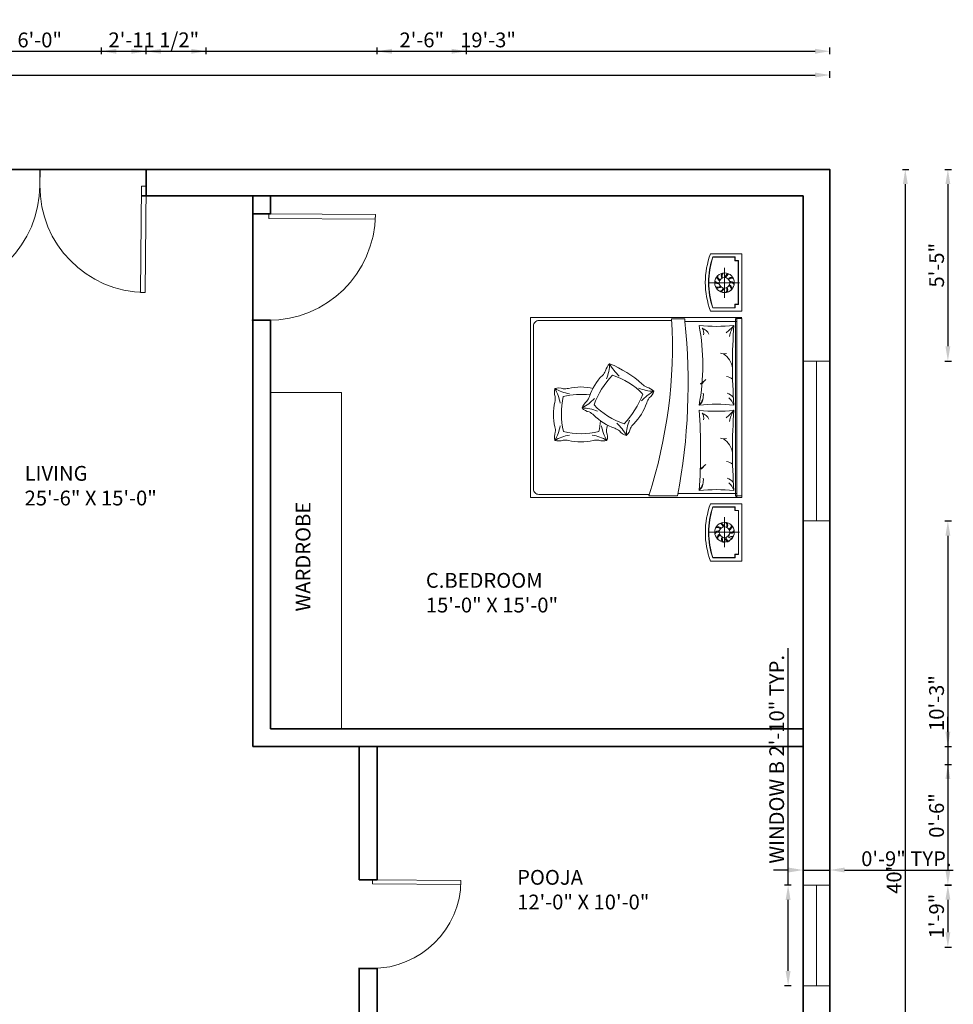
# Model space of a CAD drawing. Units: inches. Extents: x -100 to 766, y -562 to 63.
# Tile 11 of 11: x 448 to 763, y -269 to 63. Entities that reach past the tile are written whole.
import ezdxf

# ---------------------------------------------------------------- set-up
doc = ezdxf.new("R2010")
doc.units = ezdxf.units.IN
for name, color, linetype, lineweight in [('A-ANNO-DIMS', 2, 'Continuous', 18), ('A-ANNO-TEXT', 7, 'Continuous', 18), ('A-AREA-IDEN', 7, 'Continuous', 18), ('A-DOOR', 3, 'Continuous', 18), ('A-FLOR-CASE', 32, 'Continuous', 18), ('A-GLAZ', 4, 'Continuous', 18), ('A-WALL', 7, 'Continuous', 35), ('furn', 8, 'Continuous', 13)]:
    doc.layers.add(name, color=color, linetype=linetype, lineweight=lineweight)
doc.styles.get("Standard").update_dxf_attribs({"font": 'arial.ttf'})
doc.dimstyles.new('ISO-25', dxfattribs={"dimtxt": 5, "dimasz": 5, "dimexe": 1.25, "dimexo": 0.625, "dimtad": 1, "dimlunit": 3, "dimtxsty": 'Standard', "dimcen": 2.5, "dimadec": 0, "dimazin": 0, "dimtfac": 1, "dimtmove": 0, "dimatfit": 3, "dimfxl": 1, "dimfxlon": 1, "dimarcsym": 0})

# ---------------------------------------------------------------- blocks, each defined once
blk = doc.blocks.new('*U2')
for p, q in [((0, 0), (0, -6)), ((40, 0), (40, -6))]:
    blk.add_line(p, q)
blk.add_lwpolyline([(0, 0), (0, 40), (1.75, 40), (1.75, 0)], close=True)
blk.add_arc((0, 0), 40, 0, 90)
blk = doc.blocks.new('*D9')
at = {"layer": 'A-ANNO-DIMS', "color": 0, "lineweight": -2, "transparency": 16777216}
for p, q in [((1.39, 43.65), (1.39, 45.9)), ((6.39, 44.65), (716.39, 44.65)), ((721.39, 43.65), (721.39, 45.9))]:
    blk.add_line(p, q, dxfattribs=at)
at = {"layer": 'A-ANNO-DIMS', "color": 0, "transparency": 16777216}
for points in [[(6.39, 45.48), (6.39, 43.82), (1.39, 44.65)], [(716.39, 45.48), (716.39, 43.82), (721.39, 44.65)]]:
    blk.add_solid(points, dxfattribs=at)
at = {"layer": 'Defpoints', "color": 0, "transparency": 16777216}
for p in [(721.39, 44.65), (1.39, 12.79), (721.39, 12.79)]:
    blk.add_point(p, dxfattribs=at)
at = {"layer": 'A-ANNO-DIMS', "color": 0, "transparency": 16777216, "insert": (361.39, 47.83), "char_height": 5, "attachment_point": 5}
blk.add_mtext("60'", dxfattribs=at)
blk = doc.blocks.new('*D10')
at = {"layer": 'A-ANNO-DIMS', "color": 0, "lineweight": -2, "transparency": 16777216}
for p, q in [((745.89, 12.79), (748.14, 12.79)), ((746.89, 7.79), (746.89, -462.21)), ((745.89, -467.21), (748.14, -467.21))]:
    blk.add_line(p, q, dxfattribs=at)
at = {"layer": 'A-ANNO-DIMS', "color": 0, "transparency": 16777216}
for points in [[(746.06, 7.79), (747.73, 7.79), (746.89, 12.79)], [(746.06, -462.21), (747.73, -462.21), (746.89, -467.21)]]:
    blk.add_solid(points, dxfattribs=at)
at = {"layer": 'Defpoints', "color": 0, "transparency": 16777216}
for p in [(721.39, 12.79), (721.39, -467.21), (746.89, -467.21)]:
    blk.add_point(p, dxfattribs=at)
at = {"layer": 'A-ANNO-DIMS', "color": 0, "transparency": 16777216, "insert": (743.72, -227.21), "char_height": 5, "attachment_point": 5, "rotation": 90}
blk.add_mtext("40'", dxfattribs=at)
blk = doc.blocks.new('WIN-54IN')
blk.add_line((4.5, 54), (4.5, 0))
blk.add_lwpolyline([(0, 54), (9, 54), (9, 0), (0, 0)], close=True)
blk = doc.blocks.new('WIN-34IN')
blk.add_line((4.5, 34), (4.5, 0))
blk.add_lwpolyline([(0, 34), (9, 34), (9, 0), (0, 0)], close=True)
blk = doc.blocks.new('*D20')
at = {"layer": 'A-ANNO-DIMS', "color": 0, "lineweight": -2, "transparency": 16777216}
for p, q in [((707.29, -229.01), (707.29, -149.01)), ((708.29, -229.01), (706.04, -229.01)), ((707.29, -258.01), (707.29, -234.01)), ((708.29, -263.01), (706.04, -263.01))]:
    blk.add_line(p, q, dxfattribs=at)
at = {"layer": 'A-ANNO-DIMS', "color": 0, "transparency": 16777216}
for points in [[(706.45, -234.01), (708.12, -234.01), (707.29, -229.01)], [(706.45, -258.01), (708.12, -258.01), (707.29, -263.01)]]:
    blk.add_solid(points, dxfattribs=at)
at = {"layer": 'Defpoints', "color": 0, "transparency": 16777216}
for p in [(707.29, -229.01), (712.39, -229.01), (712.39, -263.01)]:
    blk.add_point(p, dxfattribs=at)
at = {"layer": 'A-ANNO-DIMS', "color": 0, "transparency": 16777216, "insert": (704.08, -186.51), "char_height": 5, "attachment_point": 5, "rotation": 90}
blk.add_mtext('WINDOW B 2\'-10" TYP.', dxfattribs=at)
blk = doc.blocks.new('*D21')
at = {"layer": 'A-ANNO-DIMS', "color": 0, "lineweight": -2, "transparency": 16777216}
for p, q in [((712.39, -224.91), (712.39, -222.66)), ((721.39, -224.91), (721.39, -222.66)), ((707.39, -223.91), (702.39, -223.91)), ((712.39, -223.91), (721.39, -223.91)), ((726.39, -223.91), (763.12, -223.91))]:
    blk.add_line(p, q, dxfattribs=at)
at = {"layer": 'A-ANNO-DIMS', "color": 0, "transparency": 16777216}
for points in [[(707.39, -223.08), (707.39, -224.75), (712.39, -223.91)], [(726.39, -223.08), (726.39, -224.75), (721.39, -223.91)]]:
    blk.add_solid(points, dxfattribs=at)
at = {"layer": 'Defpoints', "color": 0, "transparency": 16777216}
for p in [(721.39, -223.91), (712.39, -229.01), (721.39, -229.01)]:
    blk.add_point(p, dxfattribs=at)
at = {"layer": 'A-ANNO-DIMS', "color": 0, "transparency": 16777216, "insert": (747.25, -220.74), "char_height": 5, "attachment_point": 5}
blk.add_mtext('0\'-9" TYP.', dxfattribs=at)
blk = doc.blocks.new('*D44')
at = {"layer": 'A-ANNO-DIMS', "color": 0, "lineweight": -2, "transparency": 16777216}
for p, q in [((418.39, 51.68), (418.39, 53.93)), ((490.39, 51.68), (490.39, 53.93)), ((423.39, 52.68), (485.39, 52.68))]:
    blk.add_line(p, q, dxfattribs=at)
at = {"layer": 'A-ANNO-DIMS', "color": 0, "transparency": 16777216}
for points in [[(423.39, 53.51), (423.39, 51.84), (418.39, 52.68)], [(485.39, 53.51), (485.39, 51.84), (490.39, 52.68)]]:
    blk.add_solid(points, dxfattribs=at)
at = {"layer": 'Defpoints', "color": 0, "transparency": 16777216}
for p in [(490.39, 52.68), (418.39, 12.79), (490.39, 12.79)]:
    blk.add_point(p, dxfattribs=at)
at = {"layer": 'A-ANNO-DIMS', "color": 0, "transparency": 16777216, "insert": (454.39, 55.86), "char_height": 5, "attachment_point": 5}
blk.add_mtext('6\'-0"', dxfattribs=at)
blk = doc.blocks.new('*D45')
at = {"layer": 'A-ANNO-DIMS', "color": 0, "lineweight": -2, "transparency": 16777216}
for p, q in [((490.39, 51.68), (490.39, 53.93)), ((721.39, 51.68), (721.39, 53.93)), ((495.39, 52.68), (716.39, 52.68))]:
    blk.add_line(p, q, dxfattribs=at)
at = {"layer": 'A-ANNO-DIMS', "color": 0, "transparency": 16777216}
for points in [[(495.39, 53.51), (495.39, 51.84), (490.39, 52.68)], [(716.39, 53.51), (716.39, 51.84), (721.39, 52.68)]]:
    blk.add_solid(points, dxfattribs=at)
at = {"layer": 'Defpoints', "color": 0, "transparency": 16777216}
for p in [(721.39, 52.68), (490.39, 12.79), (721.39, 12.79)]:
    blk.add_point(p, dxfattribs=at)
at = {"layer": 'A-ANNO-DIMS', "color": 0, "transparency": 16777216, "insert": (605.89, 55.86), "char_height": 5, "attachment_point": 5}
blk.add_mtext('19\'-3"', dxfattribs=at)
blk = doc.blocks.new('*D48')
at = {"layer": 'A-ANNO-DIMS', "color": 0, "lineweight": -2, "transparency": 16777216}
for p, q in [((-88.51, -227.21), (-90.76, -227.21)), ((-89.51, -232.21), (-89.51, -252.21)), ((-88.51, -257.21), (-90.76, -257.21))]:
    blk.add_line(p, q, dxfattribs=at)
at = {"layer": 'A-ANNO-DIMS', "color": 0, "transparency": 16777216}
for points in [[(-90.35, -232.21), (-88.68, -232.21), (-89.51, -227.21)], [(-90.35, -252.21), (-88.68, -252.21), (-89.51, -257.21)]]:
    blk.add_solid(points, dxfattribs=at)
at = {"layer": 'Defpoints', "color": 0, "transparency": 16777216}
for p in [(562.39, -227.21), (-89.51, -257.21), (562.39, -257.21)]:
    blk.add_point(p, dxfattribs=at)
at = {"layer": 'A-ANNO-DIMS', "color": 0, "transparency": 16777216, "insert": (-92.69, -242.21), "char_height": 5, "attachment_point": 5, "rotation": 90}
blk.add_mtext('2\'-6"', dxfattribs=at)
blk = doc.blocks.new('*D52')
at = {"layer": 'A-ANNO-DIMS', "color": 0, "lineweight": -2, "transparency": 16777216}
for p, q in [((568.39, 51.68), (568.39, 53.93)), ((598.6, 51.68), (598.6, 53.93)), ((573.39, 52.68), (593.6, 52.68))]:
    blk.add_line(p, q, dxfattribs=at)
at = {"layer": 'A-ANNO-DIMS', "color": 0, "transparency": 16777216}
for points in [[(573.39, 53.51), (573.39, 51.84), (568.39, 52.68)], [(593.6, 53.51), (593.6, 51.84), (598.6, 52.68)]]:
    blk.add_solid(points, dxfattribs=at)
at = {"layer": 'Defpoints', "color": 0, "transparency": 16777216}
for p in [(598.6, 52.68), (568.39, -308.21), (598.6, -308.21)]:
    blk.add_point(p, dxfattribs=at)
at = {"layer": 'A-ANNO-DIMS', "color": 0, "transparency": 16777216, "insert": (583.5, 55.86), "char_height": 5, "attachment_point": 5}
blk.add_mtext('2\'-6"', dxfattribs=at)
blk = doc.blocks.new('*D54')
at = {"layer": 'A-ANNO-DIMS', "color": 0, "lineweight": -2, "transparency": 16777216}
for p, q in [((-88.51, -62.62), (-90.76, -62.62)), ((-89.51, -67.62), (-89.51, -171.21)), ((-88.51, -176.21), (-90.76, -176.21))]:
    blk.add_line(p, q, dxfattribs=at)
at = {"layer": 'A-ANNO-DIMS', "color": 0, "transparency": 16777216}
for points in [[(-90.35, -67.62), (-88.68, -67.62), (-89.51, -62.62)], [(-90.35, -171.21), (-88.68, -171.21), (-89.51, -176.21)]]:
    blk.add_solid(points, dxfattribs=at)
at = {"layer": 'Defpoints', "color": 0, "transparency": 16777216}
for p in [(532.39, -62.62), (-89.51, -176.21), (532.39, -176.21)]:
    blk.add_point(p, dxfattribs=at)
at = {"layer": 'A-ANNO-DIMS', "color": 0, "transparency": 16777216, "insert": (-92.72, -119.41), "char_height": 5, "attachment_point": 5, "rotation": 90}
blk.add_mtext('9\'-5 1/2"', dxfattribs=at)
blk = doc.blocks.new('*D62')
at = {"layer": 'A-ANNO-DIMS', "color": 0, "lineweight": -2, "transparency": 16777216}
for p, q in [((760.28, 12.79), (762.53, 12.79)), ((761.28, 7.79), (761.28, -46.99)), ((760.28, -51.99), (762.53, -51.99))]:
    blk.add_line(p, q, dxfattribs=at)
at = {"layer": 'A-ANNO-DIMS', "color": 0, "transparency": 16777216}
for points in [[(760.45, 7.79), (762.11, 7.79), (761.28, 12.79)], [(760.45, -46.99), (762.11, -46.99), (761.28, -51.99)]]:
    blk.add_solid(points, dxfattribs=at)
at = {"layer": 'Defpoints', "color": 0, "transparency": 16777216}
for p in [(721.39, 12.79), (721.39, -51.99), (761.28, -51.99)]:
    blk.add_point(p, dxfattribs=at)
at = {"layer": 'A-ANNO-DIMS', "color": 0, "transparency": 16777216, "insert": (758.11, -19.6), "char_height": 5, "attachment_point": 5, "rotation": 90}
blk.add_mtext('5\'-5"', dxfattribs=at)
blk = doc.blocks.new('*D63')
at = {"layer": 'A-ANNO-DIMS', "color": 0, "lineweight": -2, "transparency": 16777216}
for p, q in [((760.28, -105.99), (762.53, -105.99)), ((761.28, -110.99), (761.28, -224.01)), ((760.28, -229.01), (762.53, -229.01))]:
    blk.add_line(p, q, dxfattribs=at)
at = {"layer": 'A-ANNO-DIMS', "color": 0, "transparency": 16777216}
for points in [[(760.45, -110.99), (762.11, -110.99), (761.28, -105.99)], [(760.45, -224.01), (762.11, -224.01), (761.28, -229.01)]]:
    blk.add_solid(points, dxfattribs=at)
at = {"layer": 'Defpoints', "color": 0, "transparency": 16777216}
for p in [(721.39, -105.99), (721.39, -229.01), (761.28, -229.01)]:
    blk.add_point(p, dxfattribs=at)
at = {"layer": 'A-ANNO-DIMS', "color": 0, "transparency": 16777216, "insert": (758.1, -167.5), "char_height": 5, "attachment_point": 5, "rotation": 90}
blk.add_mtext('10\'-3"', dxfattribs=at)
blk = doc.blocks.new('*D72')
at = {"layer": 'A-ANNO-DIMS', "color": 0, "lineweight": -2, "transparency": 16777216}
for p, q in [((475.3, 51.68), (475.3, 53.93)), ((510.6, 51.68), (510.6, 53.93)), ((480.3, 52.68), (505.6, 52.68))]:
    blk.add_line(p, q, dxfattribs=at)
at = {"layer": 'A-ANNO-DIMS', "color": 0, "transparency": 16777216}
for points in [[(480.3, 53.51), (480.3, 51.84), (475.3, 52.68)], [(505.6, 53.51), (505.6, 51.84), (510.6, 52.68)]]:
    blk.add_solid(points, dxfattribs=at)
at = {"layer": 'Defpoints', "color": 0, "transparency": 16777216}
for p in [(510.6, 52.68), (475.3, -345.04), (510.6, -345.04)]:
    blk.add_point(p, dxfattribs=at)
at = {"layer": 'A-ANNO-DIMS', "color": 0, "transparency": 16777216, "insert": (492.95, 55.89), "char_height": 5, "attachment_point": 5}
blk.add_mtext('2\'-11 1/2"', dxfattribs=at)
blk = doc.blocks.new('*D74')
at = {"layer": 'A-ANNO-DIMS', "color": 0, "lineweight": -2, "transparency": 16777216}
for p, q in [((620.21, -557.16), (620.21, -559.41)), ((625.21, -558.16), (686.63, -558.16)), ((691.63, -557.16), (691.63, -559.41))]:
    blk.add_line(p, q, dxfattribs=at)
at = {"layer": 'A-ANNO-DIMS', "color": 0, "transparency": 16777216}
for points in [[(625.21, -557.32), (625.21, -558.99), (620.21, -558.16)], [(686.63, -557.32), (686.63, -558.99), (691.63, -558.16)]]:
    blk.add_solid(points, dxfattribs=at)
at = {"layer": 'Defpoints', "color": 0, "transparency": 16777216}
for p in [(620.21, -98.08), (691.63, -98.08), (691.63, -558.16)]:
    blk.add_point(p, dxfattribs=at)
at = {"layer": 'A-ANNO-DIMS', "color": 0, "transparency": 16777216, "insert": (655.92, -554.95), "char_height": 5, "attachment_point": 5}
blk.add_mtext('5\'-11 1/2"', dxfattribs=at)
blk = doc.blocks.new('*D75')
at = {"layer": 'A-ANNO-DIMS', "color": 0, "lineweight": -2, "transparency": 16777216}
for p, q in [((-88.51, -37.21), (-90.76, -37.21)), ((-89.51, -42.21), (-89.51, -93.08)), ((-88.51, -98.08), (-90.76, -98.08))]:
    blk.add_line(p, q, dxfattribs=at)
at = {"layer": 'A-ANNO-DIMS', "color": 0, "transparency": 16777216}
for points in [[(-90.35, -42.21), (-88.68, -42.21), (-89.51, -37.21)], [(-90.35, -93.08), (-88.68, -93.08), (-89.51, -98.08)]]:
    blk.add_solid(points, dxfattribs=at)
at = {"layer": 'Defpoints', "color": 0, "transparency": 16777216}
for p in [(620.21, -37.21), (-89.51, -98.08), (620.21, -98.08)]:
    blk.add_point(p, dxfattribs=at)
at = {"layer": 'A-ANNO-DIMS', "color": 0, "transparency": 16777216, "insert": (-92.69, -67.65), "char_height": 5, "attachment_point": 5, "rotation": 90}
blk.add_mtext('5\'-1"', dxfattribs=at)
blk = doc.blocks.new('*D76')
at = {"layer": 'A-ANNO-DIMS', "color": 0, "lineweight": -2, "transparency": 16777216}
for p, q in [((760.28, -228.95), (762.53, -228.95)), ((761.28, -233.95), (761.28, -244.95)), ((760.28, -249.95), (762.53, -249.95))]:
    blk.add_line(p, q, dxfattribs=at)
at = {"layer": 'A-ANNO-DIMS', "color": 0, "transparency": 16777216}
for points in [[(760.45, -233.95), (762.11, -233.95), (761.28, -228.95)], [(760.45, -244.95), (762.11, -244.95), (761.28, -249.95)]]:
    blk.add_solid(points, dxfattribs=at)
at = {"layer": 'Defpoints', "color": 0, "transparency": 16777216}
for p in [(10.38, -228.95), (10.38, -249.95), (761.28, -249.95)]:
    blk.add_point(p, dxfattribs=at)
at = {"layer": 'A-ANNO-DIMS', "color": 0, "transparency": 16777216, "insert": (758.1, -239.45), "char_height": 5, "attachment_point": 5, "rotation": 90}
blk.add_mtext('1\'-9"', dxfattribs=at)
blk = doc.blocks.new('*D82')
at = {"layer": 'A-ANNO-DIMS', "color": 0, "lineweight": -2, "transparency": 16777216}
for p, q in [((-88.51, -182.21), (-90.76, -182.21)), ((-89.51, -187.21), (-89.51, -222.21)), ((-88.51, -227.21), (-90.76, -227.21))]:
    blk.add_line(p, q, dxfattribs=at)
at = {"layer": 'A-ANNO-DIMS', "color": 0, "transparency": 16777216}
for points in [[(-90.35, -187.21), (-88.68, -187.21), (-89.51, -182.21)], [(-90.35, -222.21), (-88.68, -222.21), (-89.51, -227.21)]]:
    blk.add_solid(points, dxfattribs=at)
at = {"layer": 'Defpoints', "color": 0, "transparency": 16777216}
for p in [(562.39, -182.21), (-89.51, -227.21), (562.39, -227.21)]:
    blk.add_point(p, dxfattribs=at)
at = {"layer": 'A-ANNO-DIMS', "color": 0, "transparency": 16777216, "insert": (-92.69, -204.71), "char_height": 5, "attachment_point": 5, "rotation": 90}
blk.add_mtext('3\'-9"', dxfattribs=at)
blk = doc.blocks.new('*D84')
at = {"layer": 'A-ANNO-DIMS', "color": 0, "lineweight": -2, "transparency": 16777216}
for p, q in [((-89.51, 8.79), (-89.51, 13.79)), ((-88.51, 3.79), (-90.76, 3.79)), ((-89.51, 3.79), (-89.51, -2.21)), ((-88.51, -2.21), (-90.76, -2.21)), ((-89.51, -7.21), (-89.51, -26.76))]:
    blk.add_line(p, q, dxfattribs=at)
at = {"layer": 'A-ANNO-DIMS', "color": 0, "transparency": 16777216}
for points in [[(-90.35, 8.79), (-88.68, 8.79), (-89.51, 3.79)], [(-90.35, -7.21), (-88.68, -7.21), (-89.51, -2.21)]]:
    blk.add_solid(points, dxfattribs=at)
at = {"layer": 'Defpoints', "color": 0, "transparency": 16777216}
for p in [(526.39, 3.79), (-89.51, -2.21), (526.39, -2.21)]:
    blk.add_point(p, dxfattribs=at)
at = {"layer": 'A-ANNO-DIMS', "color": 0, "transparency": 16777216, "insert": (-92.69, -19.49), "char_height": 5, "attachment_point": 5, "rotation": 90}
blk.add_mtext('0\'-6"', dxfattribs=at)
blk = doc.blocks.new('*D85')
at = {"layer": 'A-ANNO-DIMS', "color": 0, "lineweight": -2, "transparency": 16777216}
for p, q in [((761.28, -177.21), (761.28, -172.21)), ((760.28, -182.21), (762.53, -182.21)), ((761.28, -182.21), (761.28, -188.21)), ((760.28, -188.21), (762.53, -188.21)), ((761.28, -193.21), (761.28, -212.76))]:
    blk.add_line(p, q, dxfattribs=at)
at = {"layer": 'A-ANNO-DIMS', "color": 0, "transparency": 16777216}
for points in [[(760.45, -177.21), (762.11, -177.21), (761.28, -182.21)], [(760.45, -193.21), (762.11, -193.21), (761.28, -188.21)]]:
    blk.add_solid(points, dxfattribs=at)
at = {"layer": 'Defpoints', "color": 0, "transparency": 16777216}
for p in [(130.39, -182.21), (130.39, -188.21), (761.28, -188.21)]:
    blk.add_point(p, dxfattribs=at)
at = {"layer": 'A-ANNO-DIMS', "color": 0, "transparency": 16777216, "insert": (758.1, -205.49), "char_height": 5, "attachment_point": 5, "rotation": 90}
blk.add_mtext('0\'-6"', dxfattribs=at)

msp = doc.modelspace()

# ---------------------------------------------------------------- linework, layer by layer
at = {"layer": 'A-DOOR'}
msp.add_line((454.394, 6.283), (454.394, 12.786), dxfattribs=at)
at = {"layer": 'A-FLOR-CASE'}
for p, q in [((556.388, -62.615), (532.388, -62.615)), ((556.388, -176.214), (556.388, -62.615))]:
    msp.add_line(p, q, dxfattribs=at)
at = {"layer": 'A-WALL'}
for p, q in [((490.394, 3.786), (490.394, 12.786)), ((488.753, 3.786), (526.388, 3.786)), ((526.388, 3.786), (526.388, -182.214)), ((526.388, 3.786), (532.388, 3.786)), ((532.388, 3.786), (532.388, -2.214)), ((532.388, 3.786), (712.388, 3.786)), ((712.388, 3.786), (712.388, -458.214)), ((532.388, -2.214), (526.388, -2.214)), ((532.388, -38.214), (526.388, -38.214)), ((532.388, -38.214), (532.388, -176.214)), ((532.388, -176.214), (712.388, -176.214)), ((532.388, -182.214), (526.388, -182.214)), ((532.388, -182.214), (712.388, -182.214)), ((562.394, -227.214), (562.394, -182.214)), ((568.394, -227.214), (568.394, -182.214)), ((568.394, -227.214), (562.394, -227.214)), ((562.394, -302.214), (562.394, -257.081)), ((568.394, -257.214), (562.394, -257.214)), ((568.394, -302.214), (568.394, -257.214))]:
    msp.add_line(p, q, dxfattribs=at)
msp.add_lwpolyline([(1.388, 12.786), (721.388, 12.786), (721.388, -467.214), (1.388, -467.214)], close=True, dxfattribs=at)
at = {"layer": 'furn'}
for p, q in [((685.801, -20.455), (685.801, -30.601)), ((680.728, -25.528), (690.874, -25.528)), ((689.983, -38.57), (672.41, -38.57)), ((689.458, -38.269), (689.458, -97.022)), ((689.983, -96.685), (670.125, -96.685)), ((685.8, -114.836), (685.8, -104.69)), ((680.727, -109.763), (690.873, -109.763))]:
    msp.add_line(p, q, dxfattribs=at)
for points in [[(681.073, -15.753), (691.627, -15.753), (691.627, -35.103), (681.073, -35.103, -0.1818182)], [(672.41, -37.746), (672.41, -38.57, -0.0729439), (669.955, -97.509), (660.197, -97.509, 0.0925678), (667.934, -37.746)], [(677.217, -39.912, 0.0585956), (688.974, -39.912, 0.0368889), (688.974, -66.851, 0.052163), (677.217, -66.851, 0.0931113)], [(677.217, -68.602, 0.0585956), (688.974, -68.602, 0.0366479), (688.974, -95.719, 0.052163), (677.217, -95.719, 0.0369674)], [(681.077, -119.538), (691.631, -119.538), (691.631, -100.188), (681.077, -100.188, 0.1818182)]]:
    msp.add_lwpolyline(points, format="xyb", close=True, dxfattribs=at)
for points in [[(689.411, -34.048), (681.809, -34.048, -0.167087), (681.809, -16.809), (689.411, -16.809)], [(689.411, -33.942), (681.884, -33.942, -0.1655593), (681.884, -16.914), (689.411, -16.914)], [(667.965, -38.269), (623.029, -38.269, 0.4142136), (621.27, -40.028), (621.27, -95.263, 0.4142136), (623.029, -97.022), (660.37, -97.022)], [(645.897, -58.031, 0.0912961), (646.983, -52.881, 0.0912961), (650.214, -57.036, 0.0912961)], [(647.953, -56.756, 0.1110065), (641.704, -66.805, 0.1195491), (651.871, -73.14, 0.1078134), (658.146, -63.121)], [(658.134, -63.067, 0.1218652), (647.954, -56.756, 0.1218652)], [(630.261, -66.162, 0.0912961), (628.459, -61.216, 0.0912961), (633.398, -63.034, 0.0912961)], [(656.759, -61.114, 0.0912961), (661.912, -62.183, 0.0912961), (657.768, -65.428, 0.0912961)], [(631.331, -63.992, 0.1110065), (631.342, -75.826, 0.1195491), (643.321, -75.826, 0.0332124), (643.874, -72.187)], [(642.834, -68.879, 0.0912961), (637.68, -67.81, 0.0912961), (641.825, -64.566)], [(637.68, -67.81, 0.1594612), (640.097, -69.172, -0.0762829), (641.602, -70.253, 0.1150751), (648.689, -74.67, -0.0762829), (650.322, -75.544, 0.1594612), (652.61, -77.113)], [(653.696, -71.962, 0.0912961), (652.61, -77.113, 0.0912961), (649.379, -72.957, 0.0912961)], [(633.398, -76.989, 0.0912961), (628.459, -78.807, 0.0912961), (630.261, -73.861)], [(644.247, -73.861, 0.0912961), (646.049, -78.807, 0.0912961), (641.109, -76.989, 0.0912961)], [(628.459, -78.807, 0.1594612), (631.23, -78.685, -0.0762829), (633.079, -78.807, 0.1150751), (641.429, -78.807, -0.0762829), (643.278, -78.685, 0.1594612), (646.049, -78.807)], [(689.415, -101.243), (681.813, -101.243, 0.167087), (681.813, -118.482), (689.415, -118.482)], [(689.415, -101.349), (681.888, -101.349, 0.1655593), (681.888, -118.377), (689.415, -118.377)]]:
    msp.add_lwpolyline(points, format="xyb", dxfattribs=at)
for points in [[(690.572, -18.075), (689.305, -18.075), (689.305, -16.809)], [(690.572, -17.97), (689.411, -17.97), (689.411, -16.809)], [(690.466, -17.97), (690.466, -32.887)], [(690.572, -17.97), (690.572, -32.887)], [(690.572, -32.781), (689.305, -32.781), (689.305, -34.048)], [(690.572, -32.887), (689.411, -32.887), (689.411, -34.048)], [(691.632, -37.214), (620.215, -37.214), (620.215, -98.077), (691.632, -98.077)], [(691.632, -97.509), (689.983, -97.509), (689.983, -37.566), (691.632, -37.566), (691.632, -98.077)], [(690.576, -102.51), (689.309, -102.51), (689.309, -101.243)], [(690.576, -102.404), (689.415, -102.404), (689.415, -101.243)], [(690.47, -117.321), (690.47, -102.404)], [(690.576, -117.321), (690.576, -102.404)], [(690.576, -117.216), (689.309, -117.216), (689.309, -118.482)], [(690.576, -117.321), (689.415, -117.321), (689.415, -118.482)]]:
    msp.add_lwpolyline(points, dxfattribs=at)
for centre, radius in [((685.801, -25.528), 3.314), ((685.801, -25.528), 1.796), ((685.8, -109.763), 3.314), ((685.8, -109.763), 1.796)]:
    msp.add_circle(centre, radius, dxfattribs=at)
for centre, radius, start, end in [((685.13, -23.185), 1.624, 178.30017, 238.53802), ((686.847, -23.258), 2.129, 154.17003, 200.48975), ((686.636, -23.238), 1.624, 142.30017, 202.53802), ((687.982, -24.306), 2.129, 118.17003, 164.48975), ((687.822, -24.166), 1.624, 106.30017, 166.53802), ((683.965, -23.832), 2.129, 226.17003, 272.48975), ((683.881, -24.027), 1.624, 214.30017, 274.53802), ((685.313, -23.076), 2.129, 190.17003, 236.48975), ((688.284, -25.822), 2.129, 82.17003, 128.48975), ((688.237, -25.614), 1.624, 70.30017, 130.53802), ((686.472, -27.872), 1.624, 358.30017, 58.53802), ((686.289, -27.98), 2.129, 10.17003, 56.48975), ((687.637, -27.225), 2.129, 46.17003, 92.48975), ((687.721, -27.03), 1.624, 34.30017, 94.53802), ((683.365, -25.442), 1.624, 250.30017, 310.53802), ((683.319, -25.235), 2.129, 262.17003, 308.48975), ((683.78, -26.891), 1.624, 286.30017, 346.53802), ((683.62, -26.75), 2.129, 298.17003, 344.48975), ((684.967, -27.818), 1.624, 322.30017, 22.53802), ((684.755, -27.798), 2.129, 334.17003, 20.48975), ((677.979, -31.097), 14.092, 306.49353, 321.27919), ((698.803, -46.165), 11.65, 147.53791, 167.5233), ((690.513, -38.269), 1.055, 90, 180), ((676.129, -42.514), 2.674, 346.48229, 38.55627), ((676.946, -44.543), 3.909, 24.2916, 70.9896), ((685.631, -46.637), 2.922, 245.89274, 286.11919), ((682.002, -55.101), 6.521, 6.68493, 58.3182), ((650.004, -56.16), 4.459, 132.65224, 168.89294), ((632.405, -88.541), 38.525, 48.38179, 67.76439), ((640.176, -52.549), 6.108, 315.77185, 333.2208), ((657.58, -69.778), 18.382, 135.13065, 161.38844), ((662.266, -55.377), 6.108, 225.58539, 243.03435), ((677.716, -58.706), 0.986, 263.75428, 347.21866), ((669.039, -47.841), 14.688, 306.20852, 315.08491), ((685.711, -61.695), 4.573, 51.81741, 79.89867), ((632.757, -62.402), 4.459, 164.57915, 200.81985), ((629.658, -65.511), 4.459, 69.36661, 105.60731), ((631.758, -55.253), 6.108, 265.03874, 282.4877), ((637.254, -79.118), 18.382, 76.87111, 103.12889), ((658.623, -65.194), 4.459, 42.46578, 78.70648), ((657.775, -61.004), 4.303, 307.29372, 344.09733), ((673.853, -63.417), 4.808, 314.40604, 6.83423), ((685.062, -67.479), 4.921, 40.53543, 70.35581), ((646.388, -69.953), 18.382, 167.05756, 193.31535), ((622.506, -64.535), 6.108, 347.69876, 5.14771), ((637.377, -88.186), 24.937, 83.19556, 104.02838), ((642.485, -69.525), 5.102, 128.77541, 160.35713), ((634.393, -61.897), 6.108, 323.29829, 340.74724), ((642.092, -60.197), 18.382, 315.13065, 341.38844), ((665.279, -68.078), 6.108, 143.29829, 160.74724), ((675.53, -64.315), 3.046, 303.63488, 0.84559), ((680.915, -70.549), 8.866, 24.64565, 44.15848), ((676.129, -71.204), 2.674, 346.48229, 38.55627), ((676.946, -73.233), 3.909, 24.2916, 70.9896), ((677.979, -59.787), 14.092, 306.49353, 321.27919), ((698.803, -74.855), 11.65, 147.53791, 167.5233), ((659.496, -77.426), 6.108, 135.77185, 153.2208), ((633.444, -77.721), 5.102, 160.70232, 192.28404), ((622.542, -75.527), 6.108, 355.2252, 12.67415), ((652.059, -75.431), 6.108, 167.69876, 185.14771), ((642.146, -77.493), 4.118, 341.39955, 21.57741), ((628.177, -70.013), 18.382, 347.05756, 348.7033), ((649.992, -73.934), 4.118, 309.47264, 349.6505), ((685.631, -75.327), 2.922, 245.89274, 286.11919), ((682.002, -83.791), 6.521, 6.68493, 58.3182), ((685.711, -90.385), 4.573, 51.81741, 79.89867), ((677.716, -87.396), 0.986, 263.75428, 347.21866), ((669.039, -76.531), 14.688, 306.20852, 315.08491), ((673.853, -92.107), 4.808, 314.40604, 6.83423), ((675.53, -93.005), 3.046, 303.63488, 0.84559), ((685.062, -96.169), 4.921, 40.53543, 70.35581), ((680.915, -99.239), 8.866, 24.64565, 44.15848), ((690.513, -97.022), 1.055, 180, 270), ((683.964, -111.459), 2.129, 87.51025, 133.82997), ((683.88, -111.264), 1.624, 85.46198, 145.69983), ((683.364, -109.849), 1.624, 49.46198, 109.69983), ((683.318, -110.056), 2.129, 51.51025, 97.82997), ((683.779, -108.4), 1.624, 13.46198, 73.69983), ((683.619, -108.541), 2.129, 15.51025, 61.82997), ((684.966, -107.473), 1.624, 337.46198, 37.69983), ((684.754, -107.493), 2.129, 339.51025, 25.82997), ((686.471, -107.419), 1.624, 301.46198, 1.69983), ((686.288, -107.311), 2.129, 303.51025, 349.82997), ((687.636, -108.066), 2.129, 267.51025, 313.82997), ((687.72, -108.261), 1.624, 265.46198, 325.69983), ((685.312, -112.214), 2.129, 123.51025, 169.82997), ((685.129, -112.106), 1.624, 121.46198, 181.69983), ((686.938, -112.274), 2.129, 159.51025, 205.82997), ((686.726, -112.295), 1.624, 157.46198, 217.69983), ((688.072, -111.226), 2.129, 195.51025, 241.82997), ((687.913, -111.367), 1.624, 193.46198, 253.69983), ((688.374, -109.711), 2.129, 231.51025, 277.82997), ((688.236, -109.677), 1.624, 229.46198, 289.69983)]:
    msp.add_arc(centre, radius, start, end, dxfattribs=at)

# ---------------------------------------------------------------- block references
at = {"layer": 'A-DOOR'}
for p, xscale, yscale, zscale, rotation in [((418.394, 7.383), -0.900419896884199, 0.900419896884199, 0.900419896884199, 180), ((490.35, 7.11), 0.8971966355573497, 0.8971966355573497, 0.8971966355573497, 179.5326886568227), ((531.803, -2.2), 0.9001781838093179, 0.9001781838093179, 0.9001781838093179, 269.5326886568228), ((566.874, -227.251), 0.746647067824604, 0.746647067824604, 0.746647067824604, 269.5326886568228)]:
    msp.add_blockref('*U2', p, dxfattribs=dict(at, xscale=xscale, yscale=yscale, zscale=zscale, rotation=rotation))
at = {"layer": 'A-GLAZ'}
for name, p in [('WIN-54IN', (712.388, -105.987)), ('WIN-34IN', (712.388, -263.014))]:
    msp.add_blockref(name, p, dxfattribs=at)

# ---------------------------------------------------------------- texts
at = {"layer": 'A-ANNO-TEXT', "insert": (540.887, -136.57), "char_height": 5, "attachment_point": 1, "rotation": 90}
msp.add_mtext_dynamic_manual_height_columns('WARDROBE', width=41.4154, gutter_width=12.5, heights=[0], dxfattribs=at)
at = {"layer": 'A-AREA-IDEN', "char_height": 5, "attachment_point": 1}
for s, width, insert in [('LIVING\\P25\'-6" X 15\'-0"', 76.87012, (449.291, -87.411)), ('C.BEDROOM\\P15\'-0" X 15\'-0"', 115.1566, (584.887, -123.564)), ('POOJA\\P12\'-0" X 10\'-0"', 60.29912, (615.728, -223.878))]:
    msp.add_mtext_dynamic_manual_height_columns(s, width=width, gutter_width=12.5, heights=[0], dxfattribs=dict(at, insert=insert))

# ---------------------------------------------------------------- dimensions: what is measured, and where the dimension line sits
at = {"layer": 'A-ANNO-DIMS'}
for base, p1, p2, override, picture, middle in [((510.601, 52.678), (475.3, -345.045), (510.601, -345.045), {"dimdec": 1, "dimlfac": 1, "dimrnd": 0, "dimzin": 1, "dimdsep": 46, "dimlunit": 4, "dimfrac": 2}, '*D72', (492.951, 55.888)), ((490.394, 52.678), (418.394, 12.786), (490.394, 12.786), {"dimdec": 1, "dimlfac": 1, "dimrnd": 0, "dimzin": 1, "dimdsep": 46, "dimlunit": 4, "dimfrac": 2}, '*D44', (454.394, 55.855)), ((721.388, 52.678), (490.394, 12.786), (721.388, 12.786), {"dimdec": 1, "dimlfac": 1, "dimrnd": 0, "dimzin": 1, "dimdsep": 46, "dimlunit": 4, "dimfrac": 2}, '*D45', (605.891, 55.857)), ((598.603, 52.678), (568.394, -308.214), (598.603, -308.214), {"dimdec": 1, "dimlfac": 1, "dimrnd": 0, "dimzin": 1, "dimdsep": 46, "dimlunit": 4, "dimfrac": 2}, '*D52', (583.499, 55.855)), ((721.388, 44.65), (1.388, 12.786), (721.388, 12.786), {"dimclrd": 0, "dimclre": 0, "dimclrt": 0}, '*D9', (361.388, 47.828)), ((691.632, -558.156), (620.215, -98.077), (691.632, -98.077), {"dimdec": 1, "dimlfac": 1, "dimrnd": 0, "dimzin": 1, "dimdsep": 46, "dimlunit": 4, "dimfrac": 2}, '*D74', (655.923, -554.946))]:
    dim = msp.add_linear_dim(base=base, p1=p1, p2=p2, dimstyle='ISO-25', override=override, dxfattribs=at)
    dim.commit()
    dim.dimension.update_dxf_attribs({"geometry": picture, "text_midpoint": middle})
for base, p1, p2, override, picture, middle in [((-89.513, -2.214), (526.388, 3.786), (526.388, -2.214), {"dimdec": 1, "dimlfac": 1, "dimrnd": 0, "dimzin": 1, "dimdsep": 46, "dimlunit": 4, "dimfrac": 2}, '*D84', (-92.691, -19.485)), ((746.895, -467.214), (721.388, 12.786), (721.388, -467.214), {"dimclrd": 0, "dimclre": 0, "dimclrt": 0}, '*D10', (743.717, -227.214)), ((761.28, -51.987), (721.388, 12.786), (721.388, -51.987), {"dimdec": 1, "dimlfac": 1, "dimrnd": 0, "dimzin": 1, "dimdsep": 46, "dimlunit": 4, "dimfrac": 2}, '*D62', (758.112, -19.601)), ((-89.513, -98.077), (620.215, -37.214), (620.215, -98.077), {"dimdec": 1, "dimlfac": 1, "dimrnd": 0, "dimzin": 1, "dimdsep": 46, "dimlunit": 4, "dimfrac": 2}, '*D75', (-92.691, -67.645)), ((-89.513, -176.214), (532.388, -62.615), (532.388, -176.214), {"dimdec": 1, "dimlfac": 1, "dimrnd": 0, "dimzin": 1, "dimdsep": 46, "dimlunit": 4, "dimfrac": 2}, '*D54', (-92.723, -119.415)), ((761.28, -229.014), (721.388, -105.987), (721.388, -229.014), {"dimdec": 1, "dimlfac": 1, "dimrnd": 0, "dimzin": 1, "dimdsep": 46, "dimlunit": 4, "dimfrac": 2}, '*D63', (758.1, -167.5)), ((761.28, -188.214), (130.388, -182.214), (130.388, -188.214), {"dimdec": 1, "dimlfac": 1, "dimrnd": 0, "dimzin": 1, "dimdsep": 46, "dimlunit": 4, "dimfrac": 2}, '*D85', (758.102, -205.485)), ((-89.513, -227.214), (562.394, -182.214), (562.394, -227.214), {"dimdec": 1, "dimlfac": 1, "dimrnd": 0, "dimzin": 1, "dimdsep": 46, "dimlunit": 4, "dimfrac": 2}, '*D82', (-92.693, -204.714)), ((-89.513, -257.214), (562.394, -227.214), (562.394, -257.214), {"dimdec": 1, "dimlfac": 1, "dimrnd": 0, "dimzin": 1, "dimdsep": 46, "dimlunit": 4, "dimfrac": 2}, '*D48', (-92.691, -242.214)), ((761.28, -249.949), (10.379, -228.949), (10.379, -249.949), {"dimdec": 1, "dimlfac": 1, "dimrnd": 0, "dimzin": 1, "dimdsep": 46, "dimlunit": 4, "dimfrac": 2}, '*D76', (758.102, -239.449))]:
    dim = msp.add_linear_dim(base=base, p1=p1, p2=p2, angle=90, dimstyle='ISO-25', override=override, dxfattribs=at)
    dim.commit()
    dim.dimension.update_dxf_attribs({"geometry": picture, "text_midpoint": middle})
dim = msp.add_linear_dim(base=(707.288, -229.014), p1=(712.388, -263.014), p2=(712.388, -229.014), angle=90, text='WINDOW B <> TYP.', dimstyle='ISO-25', override={"dimdec": 1, "dimlfac": 1, "dimrnd": 0, "dimzin": 1, "dimdsep": 46, "dimlunit": 4, "dimfrac": 2}, dxfattribs=at)
dim.commit()
dim.dimension.update_dxf_attribs({"geometry": '*D20', "text_midpoint": (704.076, -186.511)})
dim = msp.add_linear_dim(base=(721.388, -223.914), p1=(712.388, -229.014), p2=(721.388, -229.014), text='<> TYP.', dimstyle='ISO-25', override={"dimdec": 1, "dimlfac": 1, "dimrnd": 0, "dimzin": 1, "dimdsep": 46, "dimlunit": 4, "dimfrac": 2}, dxfattribs=at)
dim.commit()
dim.dimension.update_dxf_attribs({"geometry": '*D21', "text_midpoint": (747.251, -220.736)})

doc.saveas('drawing.dxf')
